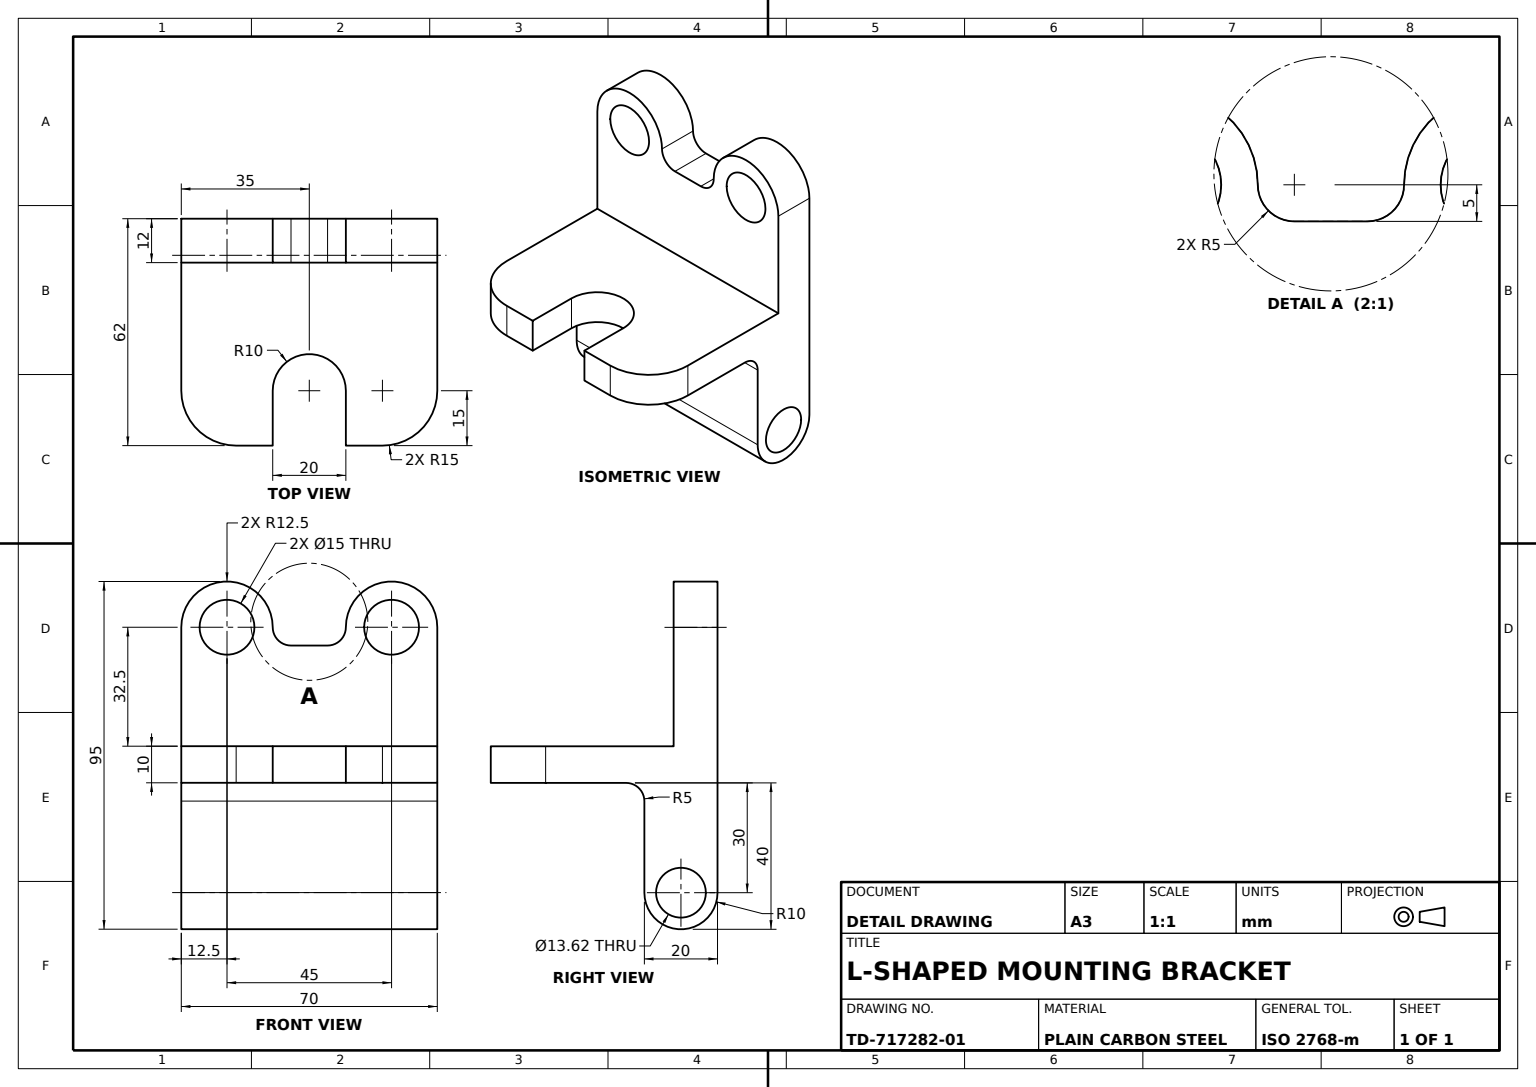
from build123d import *

# Parameters (mm, degrees)
BASE_PLATE_DEPTH      = 10
SUPPORT_BOSS_SKETCH_R = 6.810683872
SUPPORT_BOSS_DEPTH    = 70
FLANGE_DEPTH          = 12
FLANGE_SLOT_SKETCH_R  = 7.5
FLANGE_SLOT_CUT_DEPTH = 12


with BuildPart() as part:
    # Base Plate Sketch → Base Plate (new body)
    with BuildSketch(Plane(origin=(0, 0, 0), x_dir=(1, 0, 0), z_dir=(0, 1, 0))):
        with BuildLine():
            Line((0, 0), (47, 0))
            ThreePointArc((47, 0), (57.606601718, 4.393398282), (62, 15))
            Line((62, 15), (62, 25))
            Line((62, 25), (47, 25))
            ThreePointArc((47, 25), (37, 35), (47, 45))
            Line((47, 45), (62, 45))
            Line((62, 45), (62, 55))
            ThreePointArc((62, 55), (57.606601718, 65.606601718), (47, 70))
            Line((47, 70), (0, 70))
            Line((0, 70), (0, 0))
        make_face()
    extrude(amount=BASE_PLATE_DEPTH)

    # Support Boss Sketch → Support Boss (add, through all)
    with BuildSketch(Plane.XY):
        with BuildLine():
            Line((0, 0), (0, -30))
            ThreePointArc((0, -30), (10, -40), (20, -30))
            Line((20, -30), (20, -5))
            ThreePointArc((20, -5), (21.464466094, -1.464466094), (25, 0))
            Line((25, 0), (0, 0))
        make_face()
        with Locations((10, -30)):
            Circle(SUPPORT_BOSS_SKETCH_R, mode=Mode.SUBTRACT)
    extrude(amount=-SUPPORT_BOSS_DEPTH)

    # Flange Sketch → Flange (add)
    with BuildSketch(Plane.ZY):
        with BuildLine():
            Line((-70, 10), (-70, 42.5))
            ThreePointArc((-70, 42.5), (-57.5, 55), (-45, 42.5))
            ThreePointArc((-45, 42.5), (-43.535533906, 38.964466094), (-40, 37.5))
            Line((-40, 37.5), (-30, 37.5))
            ThreePointArc((-30, 37.5), (-26.464466094, 38.964466094), (-25, 42.5))
            ThreePointArc((-25, 42.5), (-12.5, 55), (0, 42.5))
            Line((0, 42.5), (0, 10))
            Line((0, 10), (-70, 10))
        make_face()
    extrude(amount=-FLANGE_DEPTH)

    # Flange Slot Sketch → Flange Slot Cut (cut)
    with BuildSketch(Plane(origin=(12, 0, 0), x_dir=(0, 0, -1), z_dir=(1, 0, 0))):
        with Locations((12.5, 42.5)):
            Circle(FLANGE_SLOT_SKETCH_R)
        with Locations((57.5, 42.5)):
            Circle(FLANGE_SLOT_SKETCH_R)
    extrude(amount=-FLANGE_SLOT_CUT_DEPTH, mode=Mode.SUBTRACT)


solid = part.part
